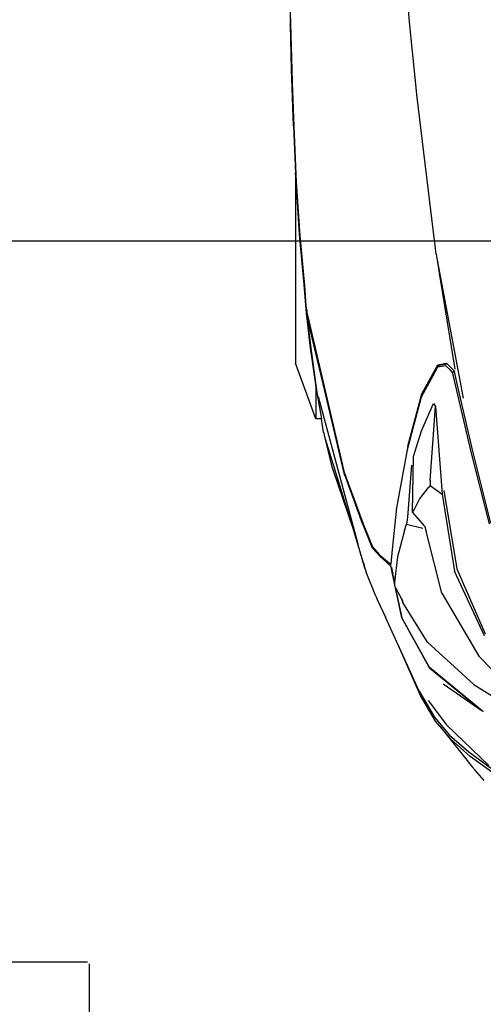
# Model space of a CAD drawing. Units: inches. Extents: x 1319 to 2030, y 219 to 1069.
# Tile 4 of 28: x 1417 to 1434, y 357 to 392. Entities that reach past the tile are written whole.
import ezdxf

# ---------------------------------------------------------------- set-up
doc = ezdxf.new("R2010")
doc.units = ezdxf.units.IN
doc.header["$MEASUREMENT"] = 0
doc.layers.get('0').update_dxf_attribs({"color": 12})
doc.layers.add('A-ANNO-DIMS', color=2, linetype='Continuous', lineweight=18)
doc.layers.add('C-PRKG-VEHC', color=8, linetype='Continuous', lineweight=13)
doc.layers.add('Edges', color=250, linetype='Continuous')
doc.styles.get("Standard").update_dxf_attribs({"font": 'arial.ttf'})
doc.dimstyles.get("Standard").update_dxf_attribs({"dimtxt": 7, "dimasz": 0.18, "dimexe": 0.18, "dimexo": 0.0625, "dimgap": 0.09, "dimtad": 0, "dimtih": 1, "dimtoh": 1, "dimzin": 0, "dimdsep": 46, "dimlunit": 3, "dimtxsty": 'Standard', "dimcen": 0.09, "dimadec": 0, "dimazin": 0, "dimtfac": 1, "dimtofl": 0, "dimtmove": 0, "dimatfit": 3, "dimfxl": 1, "dimtolj": 1, "dimtzin": 0, "dimarcsym": 0})

# ---------------------------------------------------------------- blocks, each defined once
blk = doc.blocks.new('Nissan Qashqai pl')
at = {"layer": 'Edges'}
for p, q in [((11.41698, 11.19425), (11.45295, 11.25195)), ((11.3915, 11.19885), (11.4381, 11.24397)), ((11.20627, 11.19262), (11.27199, 11.20923)), ((11.27276, 11.20843), (11.20665, 11.19145)), ((11.45306, 11.16974), (11.48975, 11.20767)), ((11.47745, 11.18983), (11.49236, 11.21027)), ((11.49628, 11.21137), (11.48154, 11.19102)), ((11.31316, 11.17892), (11.3715, 11.20434)), ((11.37334, 11.20375), (11.31527, 11.17691)), ((11.33497, 11.16556), (11.3915, 11.19885)), ((11.44046, 11.20182), (11.40144, 11.15414)), ((11.40216, 11.15476), (11.44046, 11.20182)), ((11.41633, 11.16662), (11.44046, 11.20182)), ((11.44081, 11.20225), (11.44046, 11.20182)), ((11.4411, 11.20277), (11.44081, 11.20225)), ((11.44114, 11.20281), (11.4411, 11.20277)), ((11.50327, 11.20341), (11.49363, 11.19502)), ((11.20665, 11.19145), (11.14012, 11.17593)), ((11.14803, 11.17913), (11.20627, 11.19262)), ((11.37896, 11.15265), (11.41698, 11.19425)), ((11.45433, 11.16358), (11.49082, 11.19282)), ((11.46237, 11.17248), (11.47745, 11.18983)), ((11.48154, 11.19102), (11.46617, 11.17358)), ((11.49363, 11.19502), (11.49082, 11.19282)), ((11.03575, 11.16129), (11.1598, 11.18473)), ((11.13585, 11.17654), (11.14803, 11.17913)), ((11.24278, 11.16729), (11.31316, 11.17892)), ((11.04919, 11.16347), (11.13359, 11.17719)), ((11.12846, 11.16971), (11.12929, 11.17052)), ((11.12977, 11.16183), (11.12846, 11.16971)), ((11.12929, 11.17052), (11.13526, 11.17642)), ((11.12929, 11.17052), (11.13057, 11.16299)), ((11.1347, 11.17313), (11.13062, 11.16899)), ((11.13658, 11.17502), (11.1347, 11.17313)), ((11.13526, 11.17642), (11.13585, 11.17654)), ((11.13585, 11.17654), (11.13658, 11.17502)), ((11.14012, 11.17593), (11.13658, 11.17502)), ((11.24587, 11.16563), (11.31527, 11.17691)), ((11.43143, 11.15309), (11.45306, 11.16974)), ((11.44642, 11.15882), (11.46237, 11.17248)), ((11.46617, 11.17358), (11.45433, 11.16358)), ((11.03041, 11.16033), (10.88962, 11.14337)), ((11.03041, 11.16033), (11.03575, 11.16129)), ((11.03575, 11.16129), (11.04905, 11.16345)), ((11.04919, 11.16347), (11.04905, 11.16345)), ((11.15597, 11.14759), (11.12977, 11.16183)), ((11.13192, 11.16144), (11.13057, 11.16299)), ((11.13062, 11.16899), (11.13192, 11.16144)), ((11.13192, 11.16144), (11.13652, 11.15905)), ((11.16717, 11.15976), (11.24587, 11.16563)), ((11.23823, 11.15494), (11.24587, 11.16563)), ((11.33497, 11.16556), (11.27913, 11.15147)), ((11.45433, 11.16358), (11.44983, 11.15977)), ((11.13652, 11.15905), (11.15893, 11.14704)), ((11.16444, 11.15792), (11.16717, 11.15976)), ((11.18896, 11.14734), (11.16444, 11.15792)), ((11.23369, 11.15498), (11.16717, 11.15976)), ((11.23369, 11.15498), (11.23823, 11.15494)), ((11.23823, 11.15494), (11.2401, 11.15337)), ((11.25046, 11.1455), (11.2401, 11.15337)), ((11.27429, 11.14993), (11.27913, 11.15147)), ((11.37896, 11.15265), (11.34336, 11.13032)), ((11.40144, 11.15414), (11.3571, 11.12956)), ((11.35832, 11.12998), (11.40144, 11.15414)), ((11.40216, 11.15476), (11.40144, 11.15414)), ((11.42433, 11.14593), (11.44642, 11.15882)), ((11.44983, 11.15977), (11.42671, 11.14629)), ((10.88962, 11.14337), (10.82176, 11.13649)), ((11.20291, 11.13489), (11.15597, 11.14759)), ((11.15893, 11.14704), (11.20616, 11.13437)), ((11.2121, 11.1399), (11.18896, 11.14734)), ((11.26005, 11.1405), (11.25046, 11.1455)), ((11.27429, 11.14993), (11.26224, 11.13901)), ((11.27289, 11.13379), (11.27664, 11.14845)), ((11.42671, 11.14629), (11.38067, 11.12595)), ((11.42283, 11.14525), (11.38067, 11.12595)), ((11.42283, 11.14525), (11.42433, 11.14593)), ((10.82176, 11.13649), (10.76145, 11.13107)), ((11.20291, 11.13489), (11.20295, 11.13488)), ((11.20295, 11.13488), (11.20616, 11.13437)), ((11.20616, 11.13437), (11.25827, 11.12461)), ((11.26224, 11.13901), (11.2121, 11.1399)), ((11.21991, 11.1382), (11.26663, 11.13449)), ((11.26224, 11.13901), (11.26005, 11.1405)), ((11.26663, 11.13449), (11.27289, 11.13379)), ((11.27871, 11.13184), (11.27289, 11.13379)), ((11.27871, 11.13184), (11.30218, 11.1256)), ((11.30218, 11.1256), (11.32517, 11.12286)), ((11.32955, 11.12347), (11.3571, 11.12956)), ((11.3571, 11.12956), (11.33021, 11.12384)), ((11.33021, 11.12384), (11.33938, 11.12898)), ((11.33938, 11.12898), (11.34202, 11.13045)), ((11.33938, 11.12898), (11.34336, 11.13032)), ((11.37962, 11.12547), (11.35656, 11.11477)), ((11.3571, 11.12956), (11.35832, 11.12998)), ((11.38067, 11.12595), (11.37962, 11.12547)), ((11.25827, 11.12461), (11.29558, 11.12077)), ((11.29558, 11.12077), (11.30849, 11.1195)), ((11.30003, 11.10916), (11.30813, 11.11883)), ((11.31027, 11.11923), (11.30178, 11.10961)), ((11.30805, 11.11884), (11.30863, 11.11948)), ((11.30813, 11.11883), (11.30863, 11.11948)), ((11.30849, 11.1195), (11.30863, 11.11948)), ((11.30863, 11.11948), (11.31033, 11.1193)), ((11.31033, 11.1193), (11.31027, 11.11923)), ((11.31033, 11.1193), (11.31061, 11.11927)), ((11.31061, 11.11927), (11.314, 11.12039)), ((11.31704, 11.12142), (11.31186, 11.12058)), ((11.31323, 11.11986), (11.32588, 11.12266)), ((11.32423, 11.12258), (11.314, 11.12039)), ((11.314, 11.12039), (11.31704, 11.12142)), ((11.32423, 11.12258), (11.31704, 11.12142)), ((11.31982, 11.1231), (11.32517, 11.12286)), ((11.32423, 11.12258), (11.32588, 11.12266)), ((11.32517, 11.12286), (11.32831, 11.12278)), ((11.32588, 11.12266), (11.32831, 11.12278)), ((11.32831, 11.12278), (11.32955, 11.12347)), ((11.32955, 11.12347), (11.33021, 11.12384)), ((11.29339, 11.10313), (11.30003, 11.10916)), ((11.30178, 11.10961), (11.29459, 11.10327)), ((11.33757, 11.10603), (11.34052, 11.10725)), ((11.34052, 11.10725), (11.35656, 11.11477)), ((11.29459, 11.10327), (11.27358, 11.0947)), ((11.27407, 11.09522), (11.29339, 11.10313)), ((11.33757, 11.10603), (11.31612, 11.09747)), ((11.15816, 11.05423), (11.29065, 11.08989)), ((11.2732, 11.09452), (11.22772, 11.07792)), ((11.23038, 11.07923), (11.27187, 11.09432)), ((11.27187, 11.09432), (11.27407, 11.09522)), ((11.27358, 11.0947), (11.2732, 11.09452)), ((11.27358, 11.0947), (11.27407, 11.09522)), ((11.27568, 11.08503), (11.31244, 11.09628)), ((11.31244, 11.09628), (11.29065, 11.08989)), ((11.30801, 11.09508), (11.30877, 11.09528)), ((11.31244, 11.09628), (11.31612, 11.09747)), ((11.19633, 11.06072), (11.27568, 11.08503)), ((11.22475, 11.06772), (11.27568, 11.08503)), ((11.08649, 11.04496), (11.21998, 11.07614)), ((11.22216, 11.0766), (11.08821, 11.045)), ((11.09177, 11.04531), (11.22216, 11.0766)), ((11.21998, 11.07614), (11.22216, 11.0766)), ((11.2222, 11.07656), (11.22216, 11.0766)), ((11.22715, 11.07771), (11.2222, 11.07656)), ((11.22238, 11.07665), (11.2222, 11.07656)), ((11.22238, 11.07665), (11.22532, 11.07737)), ((11.22532, 11.07737), (11.23038, 11.07923)), ((11.22731, 11.07783), (11.22706, 11.07777)), ((11.22962, 11.07837), (11.22715, 11.07771)), ((11.22772, 11.07792), (11.22715, 11.07771)), ((11.22962, 11.07837), (11.22772, 11.07792)), ((11.19297, 11.05964), (11.22148, 11.06662)), ((11.22148, 11.06662), (11.22475, 11.06772)), ((11.15472, 11.05317), (11.17828, 11.05716)), ((11.19065, 11.05923), (11.17828, 11.05716)), ((11.17828, 11.05716), (11.17828, 11.05208)), ((11.19089, 11.05929), (11.19065, 11.05923)), ((11.19089, 11.05929), (11.19297, 11.05964)), ((11.08834, 11.04438), (11.11474, 11.04762)), ((11.11234, 11.04716), (11.08834, 11.04438)), ((11.14751, 11.05208), (11.11234, 11.04716)), ((11.11474, 11.04762), (11.15472, 11.05317)), ((11.17828, 11.05208), (11.12828, 11.03408)), ((11.15248, 11.05278), (11.14751, 11.05208)), ((11.14751, 11.05208), (11.17828, 11.05208)), ((11.15472, 11.05317), (11.15248, 11.05278)), ((11.01272, 11.03746), (10.9649, 11.03441)), ((10.9657, 11.03466), (11.01381, 11.03772)), ((11.05762, 11.04159), (11.01272, 11.03746)), ((11.01381, 11.03772), (11.05899, 11.04188)), ((11.07977, 11.04339), (11.05762, 11.04159)), ((11.05899, 11.04188), (11.07681, 11.04337)), ((11.07681, 11.04337), (11.08106, 11.04371)), ((11.08696, 11.04422), (11.07977, 11.04339)), ((11.08106, 11.04371), (11.08273, 11.0441)), ((11.08114, 11.04436), (11.08208, 11.0442)), ((11.08273, 11.0441), (11.08562, 11.04476)), ((11.08273, 11.0441), (11.08365, 11.04395)), ((11.08821, 11.045), (11.08365, 11.04395)), ((11.08365, 11.04395), (11.08696, 11.04422)), ((11.08562, 11.04476), (11.08649, 11.04496)), ((11.08649, 11.04496), (11.08796, 11.04514)), ((11.08696, 11.04422), (11.08721, 11.04424)), ((11.08728, 11.04426), (11.08721, 11.04424)), ((11.08728, 11.04426), (11.08834, 11.04438)), ((10.81307, 11.02924), (10.86443, 11.03061)), ((10.81424, 11.029), (10.82415, 11.02929)), ((10.82419, 11.02929), (10.82415, 11.02929)), ((10.82464, 11.02931), (10.82419, 11.02929)), ((10.8642, 11.03037), (10.82464, 11.02931)), ((10.91525, 11.03213), (10.8642, 11.03037)), ((10.86421, 11.03053), (10.8759, 11.031)), ((10.86443, 11.03061), (10.8759, 11.031)), ((10.8759, 11.031), (10.91576, 11.03237)), ((10.91525, 11.03213), (10.95773, 11.03408)), ((10.91576, 11.03237), (10.9657, 11.03466)), ((10.9649, 11.03441), (10.95773, 11.03408)), ((10.95773, 11.03408), (11.12828, 11.03408))]:
    blk.add_line(p, q, dxfattribs=at)
blk = doc.blocks.new('car')
blk.add_blockref('Nissan Qashqai pl', (-9.74328, -11.91512))
blk = doc.blocks.new('carr')
blk.add_blockref('car', (0.51244, -0.00696))
blk = doc.blocks.new('*D56')
at = {"layer": 'A-ANNO-DIMS', "color": 0, "lineweight": -2, "transparency": 16777216}
for p, q in [((1419.852, 531.201), (1393.865, 531.201)), ((1394.045, 531.021), (1394.045, 448.679)), ((1394.045, 358.918), (1394.045, 441.26)), ((1419.852, 358.738), (1393.865, 358.738))]:
    blk.add_line(p, q, dxfattribs=at)
at = {"layer": 'A-ANNO-DIMS', "color": 0, "transparency": 16777216}
for points in [[(1394.015, 531.021), (1394.075, 531.021), (1394.045, 531.201)], [(1394.015, 358.918), (1394.075, 358.918), (1394.045, 358.738)]]:
    blk.add_solid(points, dxfattribs=at)
at = {"layer": 'Defpoints', "color": 0, "transparency": 16777216}
for p in [(1419.914, 531.201), (1394.045, 358.738), (1419.914, 358.738)]:
    blk.add_point(p, dxfattribs=at)
at = {"layer": 'A-ANNO-DIMS', "color": 0, "transparency": 16777216, "insert": (1394.045, 444.969), "char_height": 7, "attachment_point": 5}
blk.add_mtext('\\A1;CAR 14\'-4 1/2"', dxfattribs=at)
blk = doc.blocks.new('*D57')
at = {"layer": 'A-ANNO-DIMS', "color": 0, "lineweight": -2, "transparency": 16777216}
for p, q in [((1419.914, 358.675), (1419.914, 332.688)), ((1504.443, 358.675), (1504.443, 332.688)), ((1420.094, 332.868), (1444.658, 332.868)), ((1504.263, 332.868), (1479.699, 332.868))]:
    blk.add_line(p, q, dxfattribs=at)
at = {"layer": 'A-ANNO-DIMS', "color": 0, "transparency": 16777216}
for points in [[(1420.094, 332.898), (1420.094, 332.838), (1419.914, 332.868)], [(1504.263, 332.898), (1504.263, 332.838), (1504.443, 332.868)]]:
    blk.add_solid(points, dxfattribs=at)
at = {"layer": 'Defpoints', "color": 0, "transparency": 16777216}
for p in [(1419.914, 358.738), (1504.443, 358.738), (1504.443, 332.868)]:
    blk.add_point(p, dxfattribs=at)
at = {"layer": 'A-ANNO-DIMS', "color": 0, "transparency": 16777216, "insert": (1462.179, 332.868), "char_height": 7, "attachment_point": 5}
blk.add_mtext('\\A1;7\'-0 1/2"', dxfattribs=at)
blk = doc.blocks.new('*D65')
at = {"layer": 'A-ANNO-DIMS', "color": 0, "lineweight": -2, "transparency": 16777216}
for p, q in [((1648.280254, 472.227245), (1329.112754, 472.227245)), ((1329.292754, 472.047245), (1329.292754, 431.817245)), ((1329.292754, 384.407245), (1329.292754, 424.637245)), ((1648.280254, 384.227245), (1329.112754, 384.227245))]:
    blk.add_line(p, q, dxfattribs=at)
at = {"layer": 'A-ANNO-DIMS', "color": 0, "transparency": 16777216}
for points in [[(1329.262754, 472.047245), (1329.322754, 472.047245), (1329.292754, 472.227245)], [(1329.262754, 384.407245), (1329.322754, 384.407245), (1329.292754, 384.227245)]]:
    blk.add_solid(points, dxfattribs=at)
at = {"layer": 'Defpoints', "color": 0, "transparency": 16777216}
for p in [(1329.292754, 472.227245), (1648.342754, 472.227245), (1648.342754, 384.227245)]:
    blk.add_point(p, dxfattribs=at)
at = {"layer": 'A-ANNO-DIMS', "color": 0, "transparency": 16777216, "insert": (1329.292754, 428.227245), "char_height": 7, "attachment_point": 5}
blk.add_mtext('\\A1;7\'-4"', dxfattribs=at)

msp = doc.modelspace()

# ---------------------------------------------------------------- block references
at = {"layer": 'C-PRKG-VEHC', "xscale": 39.37007874015748, "yscale": 39.37007874015748, "zscale": 39.37007874015748, "rotation": 270}
msp.add_blockref('carr', (1462.179, 454.621), dxfattribs=at)

# ---------------------------------------------------------------- dimensions: what is measured, and where the dimension line sits
at = {"layer": 'A-ANNO-DIMS'}
dim = msp.add_linear_dim(base=(1394.045, 358.738), p1=(1419.914, 531.201), p2=(1419.914, 358.738), angle=270, text='CAR <>', dimstyle='Standard', override={"dimdec": 1, "dimlfac": 1, "dimrnd": 0, "dimzin": 1, "dimdsep": 46, "dimlunit": 4, "dimfrac": 2}, dxfattribs=at)
dim.commit()
dim.dimension.update_dxf_attribs({"geometry": '*D56', "text_midpoint": (1394.045, 444.969)})
dim = msp.add_linear_dim(base=(1329.293, 472.227), p1=(1648.343, 384.227), p2=(1648.343, 472.227), angle=90, dimstyle='Standard', override={"dimdec": 1, "dimlfac": 1, "dimrnd": 0, "dimzin": 1, "dimdsep": 46, "dimlunit": 4, "dimfrac": 2}, dxfattribs=at)
dim.commit()
dim.dimension.update_dxf_attribs({"geometry": '*D65', "text_midpoint": (1329.293, 428.227)})
dim = msp.add_linear_dim(base=(1504.443, 332.868), p1=(1419.914, 358.738), p2=(1504.443, 358.738), dimstyle='Standard', override={"dimdec": 1, "dimlfac": 1, "dimrnd": 0, "dimzin": 1, "dimdsep": 46, "dimlunit": 4, "dimfrac": 2}, dxfattribs=at)
dim.commit()
dim.dimension.update_dxf_attribs({"geometry": '*D57', "text_midpoint": (1462.179, 332.868)})

doc.saveas('drawing.dxf')
